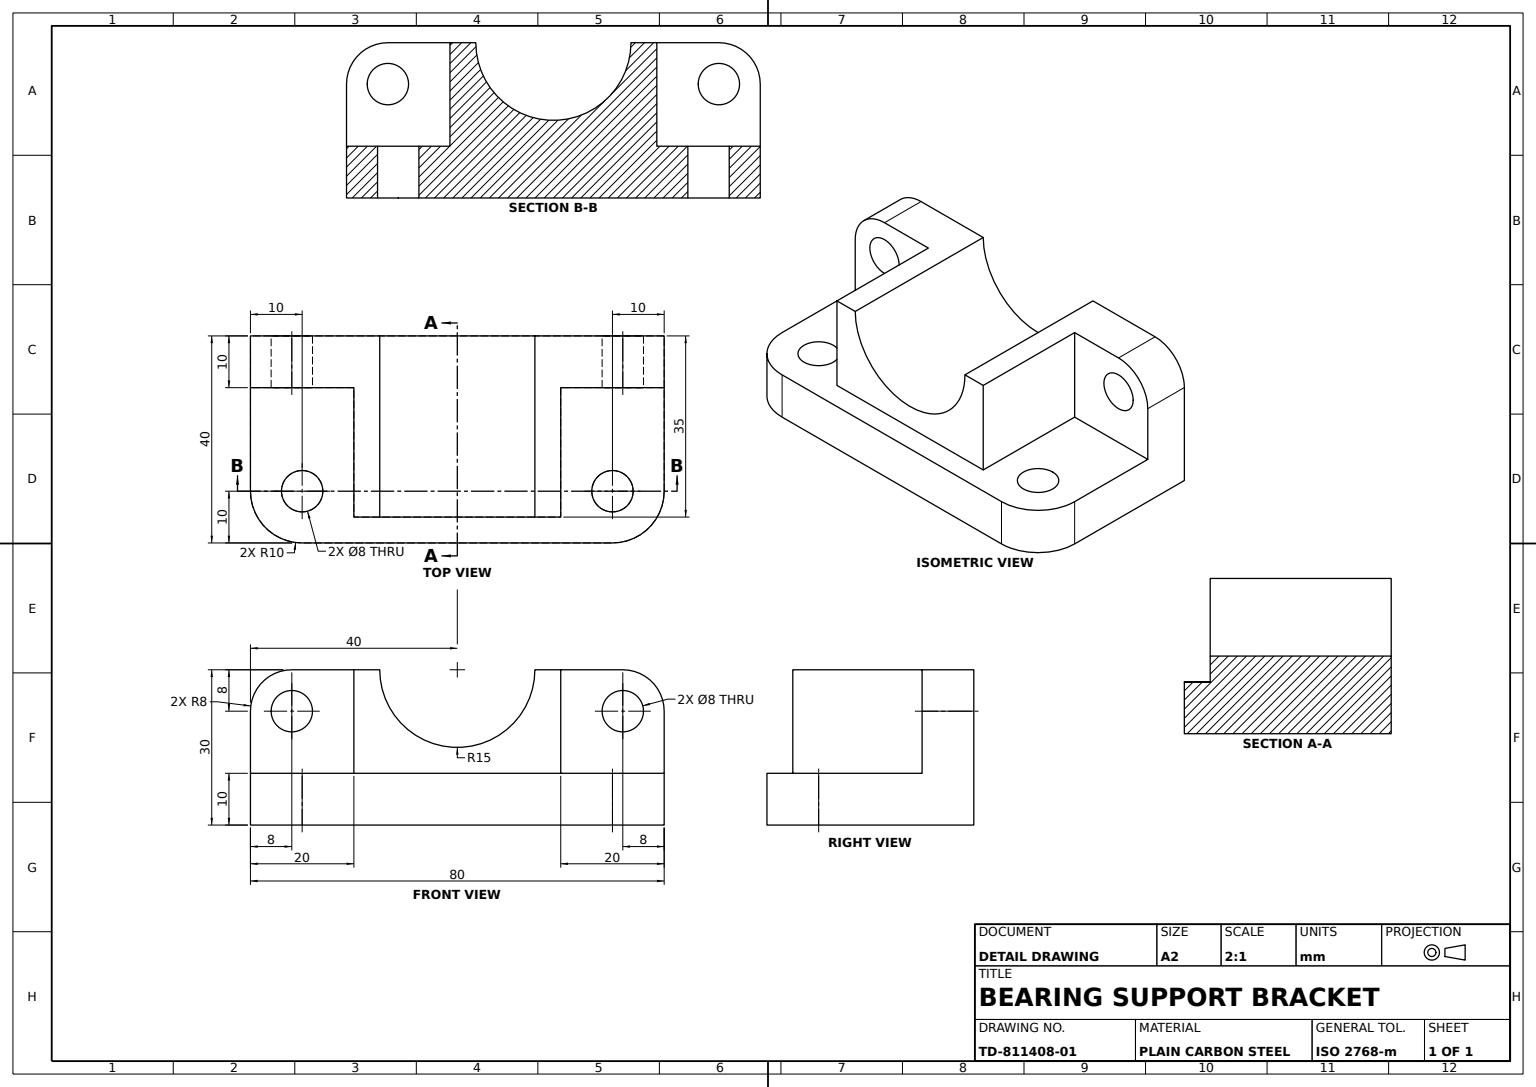
SolidWorks part; units mm, degrees
material "Plain Carbon Steel"
ref_plane "Front Plane" through (0, 0, 0) normal (0, 0, 1) x (1, 0, 0)
ref_plane "Top Plane" through (0, 0, 0) normal (0, 1, 0) x (1, 0, 0)
ref_plane "Right Plane" through (0, 0, 0) normal (1, 0, 0) x (0, 0, -1)
sketch "Base Plate Sketch" plane through (0, 0, 0) normal (0, 1, 0) x (1, 0, 0)
  line L1 (-40, 20) -> (40, 20)
  line L2 (-40, 20) -> (-40, -20)
  line L3 (-40, -20) -> (40, -20)
  line L4 (40, 20) -> (40, -20)
  line L5 (-40, 20) -> (40, -20) construction
  line L6 (-40, -20) -> (40, 20) construction
  point P0 (0, 0)
  dimension "D1" = 80
  dimension "D2" = 40
extrude "Base Plate 80x40x10" add sketch "Base Plate Sketch" along normal blind 10
fillet "Base Corner Fillets R10" radius 10 2 edges at (40, 5, 20) (-40, 5, 20)
sketch "Saddle Block Sketch" plane through (0, 0, -20) normal (0, 0, -1) x (-1, 0, 0)
  line L0 (-40, 10) -> (40, 10) construction
  line L1 (-20, 10) -> (20, 10)
  line L2 (-20, 10) -> (-20, 30)
  line L3 (-20, 30) -> (-15, 30)
  line L4 (20, 10) -> (20, 30)
  line L5 (15, 30) -> (20, 30)
  arc A0 (-15, 30) -> (15, 30) centre (0, 30) ccw
  point P6 (0, 10)
  dimension "D3" = 30
  dimension "D4" = 15
  dimension "D1" = 20
  dimension "D2" = 40
extrude "Saddle Block" add sketch "Saddle Block Sketch" against normal blind 35
sketch "Lug Profile Sketch" plane through (0, 0, -20) normal (0, 0, -1) x (-1, 0, 0)
  line L0 (20, 30) -> (15, 30) construction
  line L1 (-20, 10) -> (-40, 10)
  line L2 (-20, 10) -> (-20, 30)
  line L3 (-20, 30) -> (-40, 30)
  line L4 (-40, 10) -> (-40, 30)
  line L5 (20, 10) -> (40, 10)
  line L6 (20, 10) -> (20, 30)
  line L7 (20, 30) -> (40, 30)
  line L8 (40, 10) -> (40, 30)
  line L10 (-15, 30) -> (-20, 30) construction
  line L11 (-40, 10) -> (-40, 0) construction
  line L12 (40, 10) -> (40, 0) construction
extrude "Upright Lugs" add sketch "Lug Profile Sketch" against normal blind 10
fillet "Lug Top Fillets R8" radius 8 2 edges at (-40, 30, -15) (40, 30, -15)
sketch "Lug Hole Sketch" plane through (0, 0, -20) normal (0, 0, -1) x (-1, 0, 0)
  circle A0 centre (32, 22) radius 4
  circle A1 centre (-32, 22) radius 4
  dimension "D1" = 8
extrude "Lug Holes Ø8" cut sketch "Lug Hole Sketch" against normal blind 62
sketch "Base Hole Sketch" plane through (0, 10, 0) normal (0, 1, 0) x (1, 0, 0)
  circle A0 centre (-30, -10) radius 4
  circle A1 centre (30, -10) radius 4
  dimension "D1" = 8
extrude "Base Holes Ø8" cut sketch "Base Hole Sketch" against normal blind 62
